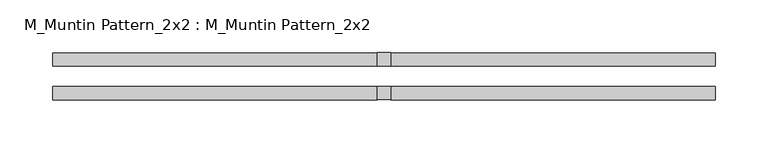
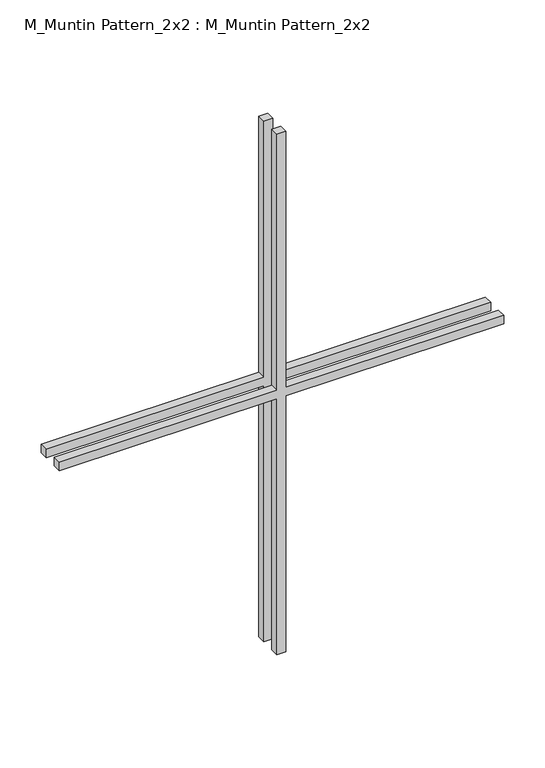
"""IFC4 building model written with IfcOpenShell, lengths in millimetres: proxy geometry, M_Muntin Pattern_2x2 : M_Muntin Pattern_2x2."""

from ifc_helpers import new_model, si_unit, frame, origin, place, context, project, spatial, polyline, outline, extrude, source, transform, mapped, element, save


def m_muntin_pattern_2x2_m_muntin_pattern_2x2_9352d081(model_context):
    return source(origin(), model_context, "Body", "SweptSolid", [
        extrude(outline(polyline([(393.7, -6.35), (393.7, -312.7375), (381.0, -312.7375), (381.0, -6.35), (0.0, -6.35), (0.0, 6.35), (381.0, 6.35), (381.0, 312.7375), (393.7, 312.7375), (393.7, 6.35), (774.7, 6.35), (774.7, -6.35), (393.7, -6.35)])), frame((0.0, 9.525, 0.0), z_axis=(0.0, 1.0, 0.0), x_axis=(0.0, 0.0, 1.0)), (0.0, 0.0, 1.0), 12.7),
        extrude(outline(polyline([(393.7, -6.35), (393.7, -312.7375), (381.0, -312.7375), (381.0, -6.35), (0.0, -6.35), (0.0, 6.35), (381.0, 6.35), (381.0, 312.7375), (393.7, 312.7375), (393.7, 6.35), (774.7, 6.35), (774.7, -6.35), (393.7, -6.35)])), frame((0.0, -22.225, 0.0), z_axis=(0.0, 1.0, 0.0), x_axis=(0.0, 0.0, 1.0)), (0.0, 0.0, 1.0), 12.7),
    ])


if __name__ == "__main__":
    model = new_model("IFC4")
    model_context = context("Model", 3, world=origin())
    ifc_project = project(units=[si_unit("LENGTHUNIT", "METRE", prefix="MILLI")], contexts=[model_context])
    site = spatial("IfcSite", under=ifc_project)
    building = spatial("IfcBuilding", under=site)
    placement = place(None, origin())
    m_muntin_pattern_2x2_m_muntin_pattern_2x2_shape = m_muntin_pattern_2x2_m_muntin_pattern_2x2_9352d081(model_context)
    element("IfcBuildingElementProxy", 1, Name="M_Muntin Pattern_2x2 : M_Muntin Pattern_2x2", ObjectType="M_Muntin Pattern_2x2 : M_Muntin Pattern_2x2", at=placement, inside=building, context=model_context, shape_type="MappedRepresentation", body=[
        mapped(m_muntin_pattern_2x2_m_muntin_pattern_2x2_shape, transform((0.0, 0.0, 0.0), x_axis=(1.0, 0.0, 0.0), y_axis=(0.0, 1.0, 0.0), z_axis=(0.0, 0.0, 1.0))),
    ])
    save(model, "model.ifc")

# Revit data of these elements
# Type "M_Muntin Pattern_2x2 : M_Muntin Pattern_2x2"
#   Width [instance default] = 3' - 11.24409"
#   Thickness = 0' - 0 1/2"
#   Height [instance default] = 3' - 11.24409"
#   Distance = 0' - 0 3/4"
#   Interior Material [instance default] = none
#   Exterior Material [instance default] = none
#   Default Elevation = 0
# Element 1 (IfcBuildingElementProxy, "M_Muntin Pattern_2x2 : M_Muntin Pattern_2x2")
#   Width = 2' - 0 5/8"
#   Height = 2' - 6 1/2"
#   Interior Material = Wood - Stained
#   Exterior Material = Clad - White
#   Materials on its faces: "Clad - White", "Wood - Stained"
# Materials
#   "Clad - White": class "Wood", colour RGB 242 242 238, transparency 0, Cost = 0
#   "Wood - Stained": class "Wood", colour RGB 224 178 126, transparency 0, Cost = 0
